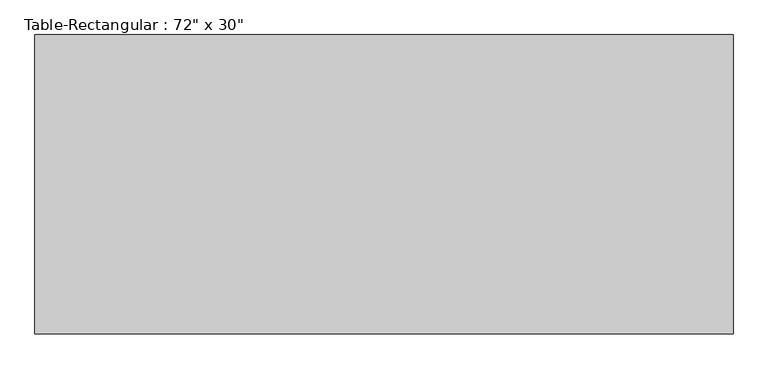
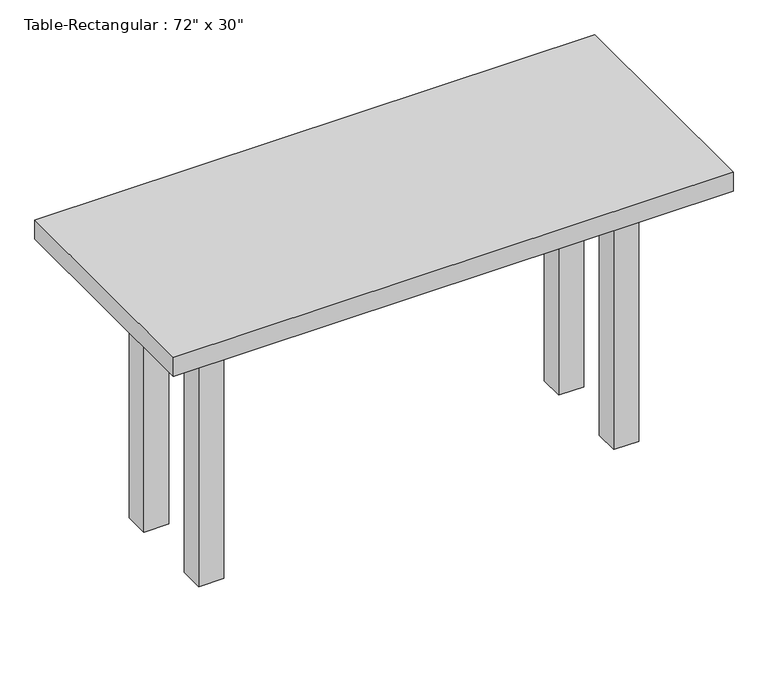
"""IFC4 building model written with IfcOpenShell, lengths in millimetres: furniture geometry."""

from ifc_helpers import new_model, si_unit, frame, origin, origin_with_axes, place, context, project, spatial, polyline, outline, extrude, source, transform, mapped, element, save


def furniture_0d1ceb4d(model_context):
    return source(origin(), model_context, "Body", "SweptSolid", [
        extrude(outline(polyline([(495.3, 114.3), (495.3, 88.9), (-495.3, 88.9), (-495.3, 114.3), (495.3, 114.3)])), frame((0.0, 0.0, 609.6), z_axis=(0.0, 0.0, 1.0), x_axis=(1.0, 0.0, 0.0)), (0.0, 0.0, 1.0), 101.6),
        extrude(outline(polyline([(495.3, -114.3), (-495.3, -114.3), (-495.3, -88.9), (495.3, -88.9), (495.3, -114.3)])), frame((0.0, 0.0, 609.6), z_axis=(0.0, 0.0, 1.0), x_axis=(1.0, 0.0, 0.0)), (0.0, 0.0, 1.0), 101.6),
        extrude(outline(polyline([(-508.0, -88.9), (-533.4, -88.9), (-533.4, 88.9), (-508.0, 88.9), (-508.0, -88.9)])), frame((0.0, 0.0, 609.6), z_axis=(0.0, 0.0, 1.0), x_axis=(1.0, 0.0, 0.0)), (0.0, 0.0, 1.0), 101.6),
        extrude(outline(polyline([(508.0, -88.9), (508.0, 88.9), (533.4, 88.9), (533.4, -88.9), (508.0, -88.9)])), frame((0.0, 0.0, 609.6), z_axis=(0.0, 0.0, 1.0), x_axis=(1.0, 0.0, 0.0)), (0.0, 0.0, 1.0), 101.6),
        extrude(outline(polyline([(711.2, 304.8), (711.2, -304.8), (-711.2, -304.8), (-711.2, 304.8), (711.2, 304.8)])), frame((0.0, 0.0, 711.2), z_axis=(0.0, 0.0, 1.0), x_axis=(1.0, 0.0, 0.0)), (0.0, 0.0, 1.0), 50.8),
        extrude(outline(polyline([(-495.3, 152.4), (-495.3, 88.9), (-558.8, 88.9), (-558.8, 152.4), (-495.3, 152.4)])), origin_with_axes(), (0.0, 0.0, 1.0), 711.2),
        extrude(outline(polyline([(495.3, 152.4), (558.8, 152.4), (558.8, 88.9), (495.3, 88.9), (495.3, 152.4)])), origin_with_axes(), (0.0, 0.0, 1.0), 711.2),
        extrude(outline(polyline([(-495.3, -152.4), (-558.8, -152.4), (-558.8, -88.9), (-495.3, -88.9), (-495.3, -152.4)])), origin_with_axes(), (0.0, 0.0, 1.0), 711.2),
        extrude(outline(polyline([(495.3, -152.4), (495.3, -88.9), (558.8, -88.9), (558.8, -152.4), (495.3, -152.4)])), origin_with_axes(), (0.0, 0.0, 1.0), 711.2),
    ])


if __name__ == "__main__":
    model = new_model("IFC4")
    model_context = context("Model", 3, world=origin())
    ifc_project = project(units=[si_unit("LENGTHUNIT", "METRE", prefix="MILLI")], contexts=[model_context])
    site = spatial("IfcSite", under=ifc_project)
    building = spatial("IfcBuilding", under=site)
    placement = place(None, origin())
    furniture_shape = furniture_0d1ceb4d(model_context)
    element("IfcFurniture", 1, ObjectType="Table-Rectangular : 72\" x 30\"", at=placement, inside=building, context=model_context, shape_type="MappedRepresentation", body=[
        mapped(furniture_shape, transform((0.0, 0.0, 0.0), x_axis=(1.0, 0.0, 0.0), y_axis=(0.0, 1.0, 0.0), z_axis=(0.0, 0.0, 1.0))),
    ])
    save(model, "model.ifc")

# Revit data of these elements
# Type "Table-Rectangular : 72\" x 30\""
#   Assembly Code = "E2020200"
#   Height = 2' - 6"
#   Length = 4' - 8"
#   Width = 2' - 0"
#   Base Material = Birch
#   Top Material = Birch
#   Default Elevation = 0
# Element 1 (IfcFurniture, "Table-Rectangular : 72\" x 30\"")
#   Materials on its faces: "Birch"
# Materials
#   "Birch": class "Wood", colour RGB 224 178 126, transparency 0, Description = "Betula Alleghaniensis", Cost = 0
